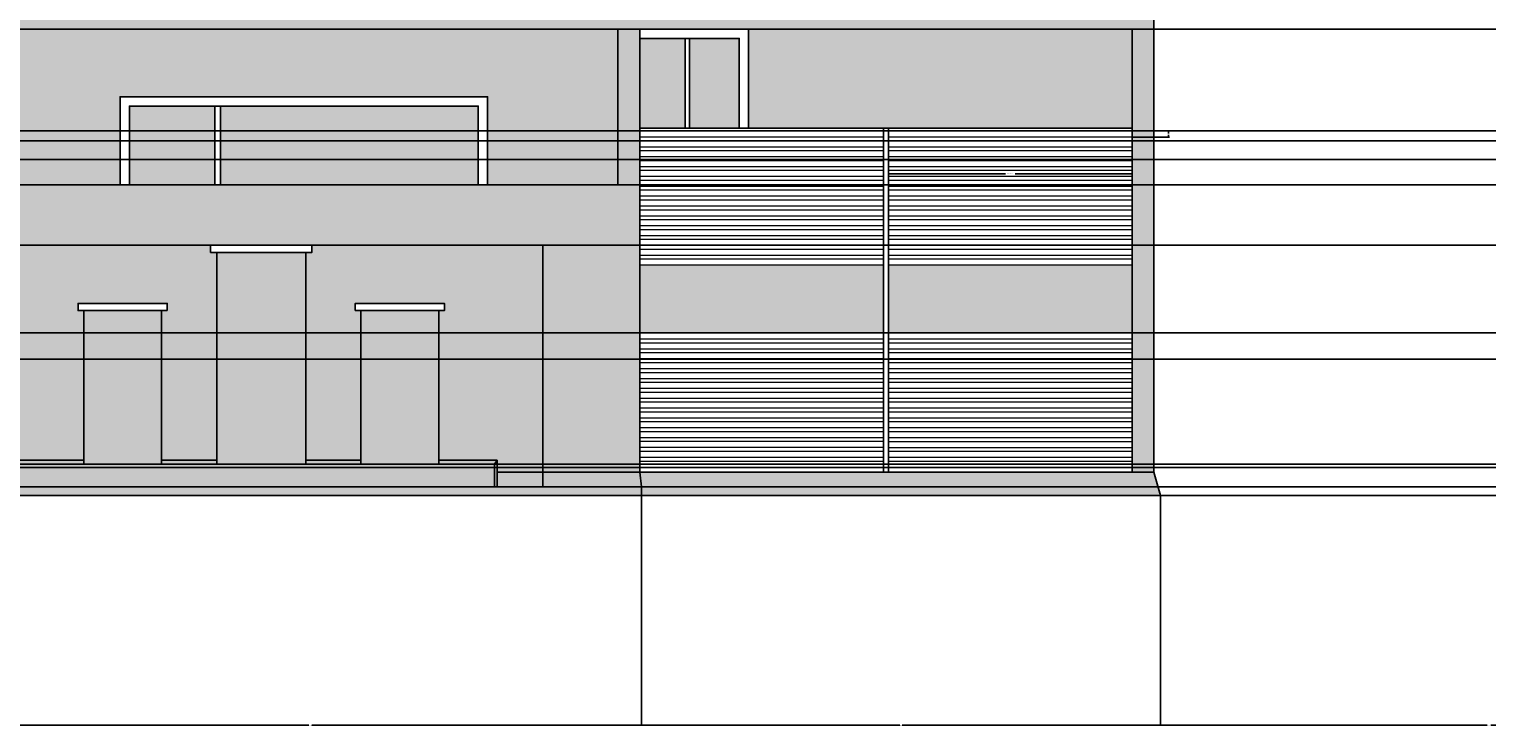
# Model space of a CAD drawing. Units: feet. Extents: x 2193 to 3502, y 890 to 1601.
# Tile 3 of 17: x 2466 to 2848, y 890 to 1073. Entities that reach past the tile are written whole.
import ezdxf

# ---------------------------------------------------------------- set-up
doc = ezdxf.new("R2010")
doc.units = ezdxf.units.FT
for name, color, linetype, lineweight in [('A-ANNO-DIMS', 2, 'Continuous', 18), ('A-ELEV', 7, 'Continuous', 25), ('A-ELEV-GATE', 4, 'Continuous', 18), ('A-ELEV-PATT', 8, 'Continuous', 13)]:
    doc.layers.add(name, color=color, linetype=linetype, lineweight=lineweight)
doc.styles.get("Standard").update_dxf_attribs({"font": 'arial.ttf'})
doc.dimstyles.get("Standard").update_dxf_attribs({"dimtxt": 0.18, "dimasz": 0.18, "dimexe": 0.18, "dimexo": 0.0625, "dimgap": 0.09, "dimtad": 0, "dimtih": 1, "dimtoh": 1, "dimdec": 0, "dimzin": 0, "dimdsep": 46, "dimlunit": 3, "dimtxsty": 'Standard', "dimcen": 0.09, "dimadec": 0, "dimazin": 0, "dimtfac": 1, "dimtdec": 0, "dimtofl": 0, "dimtmove": 0, "dimatfit": 3, "dimfxl": 1, "dimtolj": 1, "dimtzin": 0, "dimarcsym": 0})

# ---------------------------------------------------------------- blocks, each defined once
blk = doc.blocks.new('GATE-SLAT')
blk.add_lwpolyline([(0, 1.66), (63.84, 1.66), (63.84, 0), (0, 0)])
blk.add_lwpolyline([(0, 1.66), (63.84, 1.66), (63.84, 0), (0, 0)])
blk = doc.blocks.new('*D11')
at = {"layer": 'A-ANNO-DIMS', "color": 0, "lineweight": -2, "transparency": 16777216}
for p, q in [((2690.92, 1044.64), (2690.92, 1034.95)), ((2754.77, 1044.64), (2754.77, 1034.95)), ((2691.1, 1035.13), (2721.59, 1035.13)), ((2754.59, 1035.13), (2724.1, 1035.13))]:
    blk.add_line(p, q, dxfattribs=at)
at = {"layer": 'A-ANNO-DIMS', "color": 0, "transparency": 16777216}
for points in [[(2691.1, 1035.16), (2691.1, 1035.1), (2690.92, 1035.13)], [(2754.59, 1035.16), (2754.59, 1035.1), (2754.77, 1035.13)]]:
    blk.add_solid(points, dxfattribs=at)
at = {"layer": 'Defpoints', "color": 0, "transparency": 16777216}
for p in [(2690.92, 1044.7), (2754.77, 1044.7), (2754.77, 1035.13)]:
    blk.add_point(p, dxfattribs=at)
at = {"layer": 'A-ANNO-DIMS', "color": 0, "transparency": 16777216, "insert": (2722.84, 1035.13), "char_height": 0.18, "attachment_point": 5}
blk.add_mtext('\\A1;GATE SLAT 64 TYP.', dxfattribs=at)
blk = doc.blocks.new('*D12')
at = {"layer": 'A-ANNO-DIMS', "color": 0, "lineweight": -2, "transparency": 16777216}
for p, q in [((2754.83, 1046.36), (2764.52, 1046.36)), ((2754.83, 1044.7), (2764.52, 1044.7)), ((2764.34, 1046.18), (2764.34, 1045.71)), ((2764.34, 1044.88), (2764.34, 1045.35))]:
    blk.add_line(p, q, dxfattribs=at)
at = {"layer": 'A-ANNO-DIMS', "color": 0, "transparency": 16777216}
for points in [[(2764.31, 1046.18), (2764.37, 1046.18), (2764.34, 1046.36)], [(2764.31, 1044.88), (2764.37, 1044.88), (2764.34, 1044.7)]]:
    blk.add_solid(points, dxfattribs=at)
at = {"layer": 'Defpoints', "color": 0, "transparency": 16777216}
for p in [(2754.77, 1046.36), (2754.77, 1044.7), (2764.34, 1046.36)]:
    blk.add_point(p, dxfattribs=at)
at = {"layer": 'A-ANNO-DIMS', "color": 0, "transparency": 16777216, "insert": (2764.34, 1045.53), "char_height": 0.18, "attachment_point": 5}
blk.add_mtext('\\A1;2 TYP.', dxfattribs=at)
blk = doc.blocks.new('*D19')
at = {"layer": 'A-ANNO-DIMS', "color": 0, "lineweight": -2, "transparency": 16777216}
for p, q in [((2934.31, 1073.03), (2193.56, 1073.03)), ((2193.74, 1072.85), (2193.74, 1012.11)), ((2193.74, 951), (2193.74, 1011.75)), ((2934.31, 950.82), (2193.56, 950.82))]:
    blk.add_line(p, q, dxfattribs=at)
at = {"layer": 'A-ANNO-DIMS', "color": 0, "transparency": 16777216}
for points in [[(2193.71, 1072.85), (2193.77, 1072.85), (2193.74, 1073.03)], [(2193.71, 951), (2193.77, 951), (2193.74, 950.82)]]:
    blk.add_solid(points, dxfattribs=at)
at = {"layer": 'Defpoints', "color": 0, "transparency": 16777216}
for p in [(2193.74, 1073.03), (2934.37, 1073.03), (2934.37, 950.82)]:
    blk.add_point(p, dxfattribs=at)
at = {"layer": 'A-ANNO-DIMS', "color": 0, "transparency": 16777216, "insert": (2193.74, 1011.93), "char_height": 0.18, "attachment_point": 5}
blk.add_mtext('\\A1;122.2', dxfattribs=at)
blk = doc.blocks.new('*D23')
at = {"layer": 'A-ANNO-DIMS', "color": 0, "lineweight": -2, "transparency": 16777216}
for p, q in [((2988.24, 1038.87), (2193.56, 1038.87)), ((2193.74, 1038.69), (2193.74, 1012.87)), ((2193.74, 986.69), (2193.74, 1012.51)), ((2985.8, 986.51), (2193.56, 986.51))]:
    blk.add_line(p, q, dxfattribs=at)
at = {"layer": 'A-ANNO-DIMS', "color": 0, "transparency": 16777216}
for points in [[(2193.71, 1038.69), (2193.77, 1038.69), (2193.74, 1038.87)], [(2193.71, 986.69), (2193.77, 986.69), (2193.74, 986.51)]]:
    blk.add_solid(points, dxfattribs=at)
at = {"layer": 'Defpoints', "color": 0, "transparency": 16777216}
for p in [(2193.74, 1038.87), (2988.31, 1038.87), (2985.86, 986.51)]:
    blk.add_point(p, dxfattribs=at)
at = {"layer": 'A-ANNO-DIMS', "color": 0, "transparency": 16777216, "insert": (2193.74, 1012.69), "char_height": 0.18, "attachment_point": 5}
blk.add_mtext('\\A1;52.35', dxfattribs=at)
blk = doc.blocks.new('*D26')
at = {"layer": 'A-ANNO-DIMS', "color": 0, "lineweight": -2, "transparency": 16777216}
for p, q in [((2255.16, 950.89), (2255.16, 1601.47)), ((2255.34, 1601.29), (2507.42, 1601.29)), ((2760.29, 1601.29), (2508.21, 1601.29)), ((2760.47, 1541.11), (2760.47, 1601.47))]:
    blk.add_line(p, q, dxfattribs=at)
at = {"layer": 'A-ANNO-DIMS', "color": 0, "transparency": 16777216}
for points in [[(2255.34, 1601.32), (2255.34, 1601.26), (2255.16, 1601.29)], [(2760.29, 1601.32), (2760.29, 1601.26), (2760.47, 1601.29)]]:
    blk.add_solid(points, dxfattribs=at)
at = {"layer": 'Defpoints', "color": 0, "transparency": 16777216}
for p in [(2760.47, 1601.29), (2760.47, 1541.04), (2255.16, 950.82)]:
    blk.add_point(p, dxfattribs=at)
at = {"layer": 'A-ANNO-DIMS', "color": 0, "transparency": 16777216, "insert": (2507.82, 1601.29), "char_height": 0.18, "attachment_point": 5}
blk.add_mtext('\\A1;505.3', dxfattribs=at)
blk = doc.blocks.new('*D29')
at = {"layer": 'A-ANNO-DIMS', "color": 0, "lineweight": -2, "transparency": 16777216}
for p, q in [((2452.78, 956.87), (2452.78, 890.39)), ((2626.2, 950.76), (2626.2, 890.39)), ((2452.96, 890.57), (2539.1, 890.57)), ((2626.02, 890.57), (2539.87, 890.57))]:
    blk.add_line(p, q, dxfattribs=at)
at = {"layer": 'A-ANNO-DIMS', "color": 0, "transparency": 16777216}
for points in [[(2452.96, 890.6), (2452.96, 890.54), (2452.78, 890.57)], [(2626.02, 890.6), (2626.02, 890.54), (2626.2, 890.57)]]:
    blk.add_solid(points, dxfattribs=at)
at = {"layer": 'Defpoints', "color": 0, "transparency": 16777216}
for p in [(2452.78, 956.94), (2626.2, 950.82), (2626.2, 890.57)]:
    blk.add_point(p, dxfattribs=at)
at = {"layer": 'A-ANNO-DIMS', "color": 0, "transparency": 16777216, "insert": (2539.49, 890.57), "char_height": 0.18, "attachment_point": 5}
blk.add_mtext('\\A1;173.4', dxfattribs=at)
blk = doc.blocks.new('*D30')
at = {"layer": 'A-ANNO-DIMS', "color": 0, "lineweight": -2, "transparency": 16777216}
for p, q in [((2626.2, 950.76), (2626.2, 890.39)), ((2762.2, 950.76), (2762.2, 890.39)), ((2626.38, 890.57), (2693.92, 890.57)), ((2762.02, 890.57), (2694.48, 890.57))]:
    blk.add_line(p, q, dxfattribs=at)
at = {"layer": 'A-ANNO-DIMS', "color": 0, "transparency": 16777216}
for points in [[(2626.38, 890.6), (2626.38, 890.54), (2626.2, 890.57)], [(2762.02, 890.6), (2762.02, 890.54), (2762.2, 890.57)]]:
    blk.add_solid(points, dxfattribs=at)
at = {"layer": 'Defpoints', "color": 0, "transparency": 16777216}
for p in [(2626.2, 950.82), (2762.2, 950.82), (2762.2, 890.57)]:
    blk.add_point(p, dxfattribs=at)
at = {"layer": 'A-ANNO-DIMS', "color": 0, "transparency": 16777216, "insert": (2694.2, 890.57), "char_height": 0.18, "attachment_point": 5}
blk.add_mtext('\\A1;136', dxfattribs=at)
blk = doc.blocks.new('*D31')
at = {"layer": 'A-ANNO-DIMS', "color": 0, "lineweight": -2, "transparency": 16777216}
for p, q in [((2760.54, 1541.04), (3501.85, 1541.04)), ((3501.67, 1540.86), (3501.67, 1246.12)), ((3501.67, 951), (3501.67, 1245.75)), ((2762.27, 950.82), (3501.85, 950.82))]:
    blk.add_line(p, q, dxfattribs=at)
at = {"layer": 'A-ANNO-DIMS', "color": 0, "transparency": 16777216}
for points in [[(3501.64, 1540.86), (3501.7, 1540.86), (3501.67, 1541.04)], [(3501.64, 951), (3501.7, 951), (3501.67, 950.82)]]:
    blk.add_solid(points, dxfattribs=at)
at = {"layer": 'Defpoints', "color": 0, "transparency": 16777216}
for p in [(2760.47, 1541.04), (3501.67, 1541.04), (2762.2, 950.82)]:
    blk.add_point(p, dxfattribs=at)
at = {"layer": 'A-ANNO-DIMS', "color": 0, "transparency": 16777216, "insert": (3501.67, 1245.93), "char_height": 0.18, "attachment_point": 5}
blk.add_mtext('\\A1;590.2', dxfattribs=at)
blk = doc.blocks.new('*D98')
at = {"layer": 'A-ANNO-DIMS', "color": 0, "lineweight": -2, "transparency": 16777216}
for p, q in [((3111.07, 1032.19), (2193.56, 1032.19)), ((2193.74, 1032.01), (2193.74, 1024.48)), ((2193.74, 1016.58), (2193.74, 1024.11)), ((3111.07, 1016.4), (2193.56, 1016.4))]:
    blk.add_line(p, q, dxfattribs=at)
at = {"layer": 'A-ANNO-DIMS', "color": 0, "transparency": 16777216}
for points in [[(2193.71, 1032.01), (2193.77, 1032.01), (2193.74, 1032.19)], [(2193.71, 1016.58), (2193.77, 1016.58), (2193.74, 1016.4)]]:
    blk.add_solid(points, dxfattribs=at)
at = {"layer": 'Defpoints', "color": 0, "transparency": 16777216}
for p in [(2193.74, 1032.19), (3111.13, 1032.19), (3111.13, 1016.4)]:
    blk.add_point(p, dxfattribs=at)
at = {"layer": 'A-ANNO-DIMS', "color": 0, "transparency": 16777216, "insert": (2193.74, 1024.3), "char_height": 0.18, "attachment_point": 5}
blk.add_mtext('\\A1;15.793', dxfattribs=at)
blk = doc.blocks.new('*D116')
at = {"layer": 'A-ANNO-DIMS', "color": 0, "lineweight": -2, "transparency": 16777216}
for p, q in [((3140.16, 958.96), (2193.56, 958.96)), ((2193.74, 958.78), (2193.74, 956.18)), ((2193.74, 953.21), (2193.74, 955.81)), ((3140.16, 953.03), (2193.56, 953.03))]:
    blk.add_line(p, q, dxfattribs=at)
at = {"layer": 'A-ANNO-DIMS', "color": 0, "transparency": 16777216}
for points in [[(2193.71, 958.78), (2193.77, 958.78), (2193.74, 958.96)], [(2193.71, 953.21), (2193.77, 953.21), (2193.74, 953.03)]]:
    blk.add_solid(points, dxfattribs=at)
at = {"layer": 'Defpoints', "color": 0, "transparency": 16777216}
for p in [(2193.74, 958.96), (3140.22, 958.96), (3140.22, 953.03)]:
    blk.add_point(p, dxfattribs=at)
at = {"layer": 'A-ANNO-DIMS', "color": 0, "transparency": 16777216, "insert": (2193.74, 955.99), "char_height": 0.18, "attachment_point": 5}
blk.add_mtext('\\A1;5.924', dxfattribs=at)
blk = doc.blocks.new('*D124')
at = {"layer": 'A-ANNO-DIMS', "color": 0, "lineweight": -2, "transparency": 16777216}
for p, q in [((3304.91, 1046.36), (2193.56, 1046.36)), ((3304.91, 1043.78), (2193.56, 1043.78)), ((2193.74, 1046.18), (2193.74, 1045.26)), ((2193.74, 1043.96), (2193.74, 1044.89))]:
    blk.add_line(p, q, dxfattribs=at)
at = {"layer": 'A-ANNO-DIMS', "color": 0, "transparency": 16777216}
for points in [[(2193.71, 1046.18), (2193.77, 1046.18), (2193.74, 1046.36)], [(2193.71, 1043.96), (2193.77, 1043.96), (2193.74, 1043.78)]]:
    blk.add_solid(points, dxfattribs=at)
at = {"layer": 'Defpoints', "color": 0, "transparency": 16777216}
for p in [(2193.74, 1043.78), (3304.97, 1046.36), (3304.97, 1043.78)]:
    blk.add_point(p, dxfattribs=at)
at = {"layer": 'A-ANNO-DIMS', "color": 0, "transparency": 16777216, "insert": (2193.74, 1045.07), "char_height": 0.18, "attachment_point": 5}
blk.add_mtext('\\A1;2.583', dxfattribs=at)
blk = doc.blocks.new('*D126')
at = {"layer": 'A-ANNO-DIMS', "color": 0, "lineweight": -2, "transparency": 16777216}
for p, q in [((2762.2, 950.76), (2762.2, 890.39)), ((2934.37, 950.76), (2934.37, 890.39)), ((2762.38, 890.57), (2847.83, 890.57)), ((2934.19, 890.57), (2848.74, 890.57))]:
    blk.add_line(p, q, dxfattribs=at)
at = {"layer": 'A-ANNO-DIMS', "color": 0, "transparency": 16777216}
for points in [[(2762.38, 890.6), (2762.38, 890.54), (2762.2, 890.57)], [(2934.19, 890.6), (2934.19, 890.54), (2934.37, 890.57)]]:
    blk.add_solid(points, dxfattribs=at)
at = {"layer": 'Defpoints', "color": 0, "transparency": 16777216}
for p in [(2762.2, 950.82), (2934.37, 950.82), (2934.37, 890.57)]:
    blk.add_point(p, dxfattribs=at)
at = {"layer": 'A-ANNO-DIMS', "color": 0, "transparency": 16777216, "insert": (2848.29, 890.57), "char_height": 0.18, "attachment_point": 5}
blk.add_mtext('\\A1;172.17', dxfattribs=at)
blk = doc.blocks.new('*D130')
at = {"layer": 'A-ANNO-DIMS', "color": 0, "lineweight": -2, "transparency": 16777216}
for p, q in [((3304.91, 993.39), (2193.56, 993.39)), ((2193.74, 993.21), (2193.74, 975.95)), ((2193.74, 958.33), (2193.74, 975.59)), ((3304.91, 958.15), (2193.56, 958.15))]:
    blk.add_line(p, q, dxfattribs=at)
at = {"layer": 'A-ANNO-DIMS', "color": 0, "transparency": 16777216}
for points in [[(2193.71, 993.21), (2193.77, 993.21), (2193.74, 993.39)], [(2193.71, 958.33), (2193.77, 958.33), (2193.74, 958.15)]]:
    blk.add_solid(points, dxfattribs=at)
at = {"layer": 'Defpoints', "color": 0, "transparency": 16777216}
for p in [(2193.74, 993.39), (3304.97, 993.39), (3304.97, 958.15)]:
    blk.add_point(p, dxfattribs=at)
at = {"layer": 'A-ANNO-DIMS', "color": 0, "transparency": 16777216, "insert": (2193.74, 975.77), "char_height": 0.18, "attachment_point": 5}
blk.add_mtext('\\A1;35.24', dxfattribs=at)

msp = doc.modelspace()

# ---------------------------------------------------------------- hatches: boundary and pattern name
at = {"layer": 'A-ELEV-PATT'}
h = msp.add_hatch(color=256, dxfattribs=at)
h.dxf.hatch_style = 1
h.paths.add_polyline_path([(2760.4733, 1541.0441), (2699.6322, 1541.0441), (2699.6322, 1512.3957), (2760.4733, 1512.3957)])
h.paths.add_polyline_path([(2760.4733, 1502.0763), (2699.6322, 1502.0763), (2699.6322, 1382.0763), (2760.4733, 1382.0763)])
h.paths.add_polyline_path([(2745.971, 1367.5739), (2699.6322, 1367.5739), (2699.6322, 1089.3627), (2760.4733, 1089.3627), (2760.4733, 1166.2327), (2745.971, 1166.2327)])
h.paths.add_polyline_path([(2754.7661, 1011.1246), (2690.9216, 1011.1246), (2690.9216, 993.3923), (2754.7661, 993.3923)])
h.paths.add_polyline_path([(2689.6008, 1011.1246), (2625.7563, 1011.1246), (2625.7563, 993.3923), (2689.6008, 993.3923)])
h.paths.add_polyline_path([(2599.6883, 1249.8256), (2598.591, 1249.8256), (2598.591, 1233.561), (2599.6883, 1233.561)])
h.paths.add_polyline_path([(2602.5204, 1247.0422), (2601.423, 1247.0422), (2601.423, 1233.561), (2602.5204, 1233.561)])
h.paths.add_polyline_path([(2606.5316, 1250.4403), (2605.4342, 1250.4403), (2605.4342, 1233.561), (2606.5316, 1233.561)])
h.paths.add_polyline_path([(2609.5836, 1248.4363), (2608.4862, 1248.4363), (2608.4862, 1233.561), (2609.5836, 1233.561)])
h.paths.add_polyline_path([(2613.8564, 1243.2956), (2612.759, 1243.2956), (2612.759, 1233.561), (2613.8564, 1233.561)])
h.paths.add_polyline_path([(2616.5596, 1249.6561), (2615.4622, 1249.6561), (2615.4622, 1233.561), (2616.5596, 1233.561)])
h.paths.add_polyline_path([(2599.6883, 1233.561), (2598.591, 1233.561), (2598.591, 1224.865), (2599.6883, 1224.865)])
h.paths.add_polyline_path([(2602.5204, 1233.561), (2601.423, 1233.561), (2601.423, 1224.865), (2602.5204, 1224.865)])
h.paths.add_polyline_path([(2606.5316, 1233.561), (2605.4342, 1233.561), (2605.4342, 1224.865), (2606.5316, 1224.865)])
h.paths.add_polyline_path([(2609.5836, 1233.561), (2608.4862, 1233.561), (2608.4862, 1224.865), (2609.5836, 1224.865)])
h.paths.add_polyline_path([(2613.8564, 1233.561), (2612.759, 1233.561), (2612.759, 1224.865), (2613.8564, 1224.865)])
h.paths.add_polyline_path([(2616.5596, 1233.561), (2615.4622, 1233.561), (2615.4622, 1224.865), (2616.5596, 1224.865)])
h.paths.add_polyline_path([(2599.6883, 1224.865), (2598.591, 1224.865), (2598.591, 1115.2331), (2599.6883, 1115.2331)])
h.paths.add_polyline_path([(2602.5204, 1224.865), (2601.423, 1224.865), (2601.423, 1112.4498), (2602.5204, 1112.4498)])
h.paths.add_polyline_path([(2606.5316, 1224.865), (2605.4342, 1224.865), (2605.4342, 1115.8479), (2606.5316, 1115.8479)])
h.paths.add_polyline_path([(2609.5836, 1224.865), (2608.4862, 1224.865), (2608.4862, 1113.8439), (2609.5836, 1113.8439)])
h.paths.add_polyline_path([(2616.5596, 1224.865), (2615.4622, 1224.865), (2615.4622, 1115.0637), (2616.5596, 1115.0637)])
h.paths.add_polyline_path([(2613.8564, 1224.865), (2612.759, 1224.865), (2612.759, 1108.7032), (2613.8564, 1108.7032)])
h = msp.add_hatch(color=256, dxfattribs=at)
h.dxf.hatch_style = 1
h.paths.add_polyline_path([(2390.8933, 1367.5739), (2294.8992, 1367.5739), (2294.8992, 1329.5765), (2390.8933, 1329.5765)])
h.paths.add_polyline_path([(2489.6169, 1055.3069), (2585.8844, 1055.3069), (2585.8844, 1032.1935), (2620.0491, 1032.1935), (2620.0491, 1073.031), (2452.7821, 1073.031), (2452.7821, 1032.1935), (2489.6169, 1032.1935)])
h.paths.add_polyline_path([(2754.7661, 1073.031), (2654.2841, 1073.031), (2654.2841, 1047.0961), (2754.7661, 1047.0961)])
h.paths.add_polyline_path([(2643.9681, 1484.1152), (2699.5726, 1484.1152), (2699.5726, 1502.0763), (2602.8648, 1502.0763), (2602.8648, 1408.4814), (2643.9681, 1408.4814)])
h.paths.add_polyline_path([(2699.6322, 1367.5739), (2646.2844, 1367.5739), (2646.2844, 1268.6599), (2647.1841, 1268.6599), (2647.1841, 1329.5765), (2699.6322, 1329.5765)])
h.paths.add_polyline_path([(2699.6322, 1224.865), (2616.5596, 1224.865), (2616.5596, 1133.8558), (2647.1841, 1133.8558), (2647.1841, 1194.7724), (2699.6322, 1194.7724)])
h = msp.add_hatch(color=256, dxfattribs=at)
h.dxf.hatch_style = 1
h.paths.add_polyline_path([(2760.4733, 956.8829), (2754.7661, 956.8829), (2625.7563, 956.8829), (2626.1971, 953.031), (2626.1971, 950.8228), (2762.2048, 950.8228)])
h.paths.add_polyline_path([(2587.7084, 958.9555), (2461.0056, 958.9555), (2461.0056, 953.031), (2587.7084, 953.031)])
h.paths.add_polyline_path([(2480.0809, 960.0129), (2463.2716, 960.0129), (2461.0056, 958.9555), (2480.0809, 958.9555)])
h.paths.add_polyline_path([(2514.917, 960.0129), (2500.4779, 960.0129), (2500.4779, 958.9555), (2514.917, 958.9555)])
h.paths.add_polyline_path([(2552.6959, 960.0129), (2538.2568, 960.0129), (2538.2568, 958.9555), (2552.6959, 958.9555)])
h.paths.add_polyline_path([(2588.4279, 960.0129), (2573.0929, 960.0129), (2573.0929, 958.9555), (2587.7084, 958.9555)])
h.paths.add_polyline_path([(2588.4279, 960.0129), (2587.7084, 958.9555), (2587.7084, 953.031), (2588.4279, 953.031)])
h.paths.add_polyline_path([(2461.0056, 956.8829), (2261.443, 956.8829), (2255.1574, 953.031), (2461.0056, 953.031)])
h.paths.add_polyline_path([(2625.7563, 956.8829), (2600.3918, 956.8829), (2600.3918, 953.031), (2626.1971, 953.031)])
h.paths.add_polyline_path([(2600.3918, 956.8829), (2588.4279, 956.8829), (2588.4279, 953.031), (2600.3918, 953.031)])
h.paths.add_polyline_path([(2602.8648, 1494.8043), (2286.5029, 1494.8043), (2286.5029, 1492.5146), (2602.8648, 1492.5146)])
h.paths.add_polyline_path([(2322.8578, 1492.5146), (2319.4392, 1492.5146), (2337.7496, 1475.8561), (2341.1681, 1475.8561)])
h.paths.add_polyline_path([(2341.1681, 1475.8561), (2337.7496, 1475.8561), (2341.051, 1472.8525), (2344.4696, 1472.8525)])
h.paths.add_polyline_path([(2344.4696, 1472.8525), (2341.051, 1472.8525), (2352.3124, 1462.6071), (2355.731, 1462.6071)])
h.paths.add_polyline_path([(2355.731, 1462.6071), (2352.3124, 1462.6071), (2355.6139, 1459.6035), (2359.0325, 1459.6035)])
h.paths.add_polyline_path([(2325.1721, 1459.1592), (2323.1659, 1459.1592), (2323.1659, 1408.4814), (2325.1721, 1408.4814)])
h.paths.add_polyline_path([(2297.6937, 1482.3334), (2295.7368, 1484.1138), (2295.7368, 1408.4814), (2297.6937, 1408.4814)])
h.paths.add_polyline_path([(2300.8766, 1479.4377), (2297.6937, 1482.3334), (2297.6937, 1408.4814), (2300.8766, 1408.4814)])
h.paths.add_polyline_path([(2337.7496, 1475.8561), (2304.8133, 1475.8561), (2308.1148, 1472.8525), (2341.051, 1472.8525)])
h.paths.add_polyline_path([(2352.3124, 1462.6071), (2319.3762, 1462.6071), (2322.6776, 1459.6035), (2355.6139, 1459.6035)])
h.paths.add_polyline_path([(2374.1044, 1475.8561), (2341.1681, 1475.8561), (2344.4696, 1472.8525), (2377.4059, 1472.8525)])
h.paths.add_polyline_path([(2388.6672, 1462.6071), (2355.731, 1462.6071), (2359.0325, 1459.6035), (2391.9687, 1459.6035)])
h.paths.add_polyline_path([(2392.0858, 1462.6071), (2388.6672, 1462.6071), (2391.9687, 1459.6035), (2395.3873, 1459.6035)])
h.paths.add_polyline_path([(2380.8245, 1472.8525), (2377.4059, 1472.8525), (2388.6672, 1462.6071), (2392.0858, 1462.6071)])
h.paths.add_polyline_path([(2377.523, 1475.8561), (2374.1044, 1475.8561), (2377.4059, 1472.8525), (2380.8245, 1472.8525)])
h.paths.add_polyline_path([(2359.2126, 1492.5146), (2355.794, 1492.5146), (2374.1044, 1475.8561), (2377.523, 1475.8561)])
h.paths.add_polyline_path([(2395.5674, 1492.5146), (2392.1488, 1492.5146), (2410.4592, 1475.8561), (2413.8778, 1475.8561)])
h.paths.add_polyline_path([(2410.4592, 1475.8561), (2377.523, 1475.8561), (2380.8245, 1472.8525), (2413.7607, 1472.8525)])
h.paths.add_polyline_path([(2413.8778, 1475.8561), (2410.4592, 1475.8561), (2413.7607, 1472.8525), (2417.1793, 1472.8525)])
h.paths.add_polyline_path([(2417.1793, 1472.8525), (2413.7607, 1472.8525), (2425.022, 1462.6071), (2428.4406, 1462.6071)])
h.paths.add_polyline_path([(2425.022, 1462.6071), (2392.0858, 1462.6071), (2395.3873, 1459.6035), (2428.3235, 1459.6035)])
h.paths.add_polyline_path([(2428.4406, 1462.6071), (2425.022, 1462.6071), (2428.3235, 1459.6035), (2431.7421, 1459.6035)])
h.paths.add_polyline_path([(2461.3769, 1462.6071), (2428.4406, 1462.6071), (2431.7421, 1459.6035), (2464.6784, 1459.6035)])
h.paths.add_polyline_path([(2577.3415, 1492.5146), (2573.9229, 1492.5146), (2591.9256, 1476.1361), (2593.2177, 1478.0707)])
h.paths.add_polyline_path([(2540.9867, 1492.5146), (2537.5681, 1492.5146), (2555.8785, 1475.8561), (2559.2971, 1475.8561)])
h.paths.add_polyline_path([(2591.7386, 1475.8561), (2559.2971, 1475.8561), (2562.5986, 1472.8525), (2589.7325, 1472.8525)])
h.paths.add_polyline_path([(2555.8785, 1475.8561), (2522.9423, 1475.8561), (2526.2437, 1472.8525), (2559.18, 1472.8525)])
h.paths.add_polyline_path([(2559.2971, 1475.8561), (2555.8785, 1475.8561), (2559.18, 1472.8525), (2562.5986, 1472.8525)])
h.paths.add_polyline_path([(2562.5986, 1472.8525), (2559.18, 1472.8525), (2570.4413, 1462.6071), (2573.8599, 1462.6071)])
h.paths.add_polyline_path([(2570.4413, 1462.6071), (2537.5051, 1462.6071), (2540.8066, 1459.6035), (2573.7428, 1459.6035)])
h.paths.add_polyline_path([(2582.8896, 1462.6071), (2573.8599, 1462.6071), (2577.1614, 1459.6035), (2580.8835, 1459.6035)])
h.paths.add_polyline_path([(2573.8599, 1462.6071), (2570.4413, 1462.6071), (2573.7428, 1459.6035), (2577.1614, 1459.6035)])
h.paths.add_polyline_path([(2591.7386, 1475.8561), (2589.7325, 1472.8525), (2589.7325, 1408.4814), (2591.7386, 1408.4814)])
h.paths.add_polyline_path([(2582.8896, 1462.6071), (2580.8835, 1459.6035), (2580.8835, 1408.4814), (2582.8896, 1408.4814)])
h.paths.add_polyline_path([(2504.6319, 1492.5146), (2501.2133, 1492.5146), (2519.5237, 1475.8561), (2522.9423, 1475.8561)])
h.paths.add_polyline_path([(2534.0865, 1462.6071), (2501.1503, 1462.6071), (2504.4518, 1459.6035), (2537.388, 1459.6035)])
h.paths.add_polyline_path([(2537.5051, 1462.6071), (2534.0865, 1462.6071), (2537.388, 1459.6035), (2540.8066, 1459.6035)])
h.paths.add_polyline_path([(2526.2437, 1472.8525), (2522.8252, 1472.8525), (2534.0865, 1462.6071), (2537.5051, 1462.6071)])
h.paths.add_polyline_path([(2522.9423, 1475.8561), (2519.5237, 1475.8561), (2522.8252, 1472.8525), (2526.2437, 1472.8525)])
h.paths.add_polyline_path([(2519.5237, 1475.8561), (2486.5874, 1475.8561), (2489.8889, 1472.8525), (2522.8252, 1472.8525)])
h.paths.add_polyline_path([(2483.1689, 1475.8561), (2450.2326, 1475.8561), (2453.5341, 1472.8525), (2486.4703, 1472.8525)])
h.paths.add_polyline_path([(2486.5874, 1475.8561), (2483.1689, 1475.8561), (2486.4703, 1472.8525), (2489.8889, 1472.8525)])
h.paths.add_polyline_path([(2468.277, 1492.5146), (2464.8585, 1492.5146), (2483.1689, 1475.8561), (2486.5874, 1475.8561)])
h.paths.add_polyline_path([(2489.8889, 1472.8525), (2486.4703, 1472.8525), (2497.7317, 1462.6071), (2501.1503, 1462.6071)])
h.paths.add_polyline_path([(2497.7317, 1462.6071), (2464.7955, 1462.6071), (2468.0969, 1459.6035), (2501.0332, 1459.6035)])
h.paths.add_polyline_path([(2501.1503, 1462.6071), (2497.7317, 1462.6071), (2501.0332, 1459.6035), (2504.4518, 1459.6035)])
h.paths.add_polyline_path([(2464.7955, 1462.6071), (2461.3769, 1462.6071), (2464.6784, 1459.6035), (2468.0969, 1459.6035)])
h.paths.add_polyline_path([(2453.5341, 1472.8525), (2450.1155, 1472.8525), (2461.3769, 1462.6071), (2464.7955, 1462.6071)])
h.paths.add_polyline_path([(2431.9222, 1492.5146), (2428.5036, 1492.5146), (2446.814, 1475.8561), (2450.2326, 1475.8561)])
h.paths.add_polyline_path([(2446.814, 1475.8561), (2413.8778, 1475.8561), (2417.1793, 1472.8525), (2450.1155, 1472.8525)])
h.paths.add_polyline_path([(2450.2326, 1475.8561), (2446.814, 1475.8561), (2450.1155, 1472.8525), (2453.5341, 1472.8525)])
h.paths.add_polyline_path([(2407.5925, 1459.1592), (2405.5863, 1459.1592), (2405.5863, 1408.4814), (2407.5925, 1408.4814)])
h.paths.add_polyline_path([(2499.2252, 1459.1592), (2497.2191, 1459.1592), (2497.2191, 1408.4814), (2499.2252, 1408.4814)])
h = msp.add_hatch(color=256, dxfattribs=at)
h.dxf.hatch_style = 1
h.paths.add_polyline_path([(2294.8992, 1367.5739), (2275.0482, 1367.5739), (2275.0482, 1382.0763), (2536.5416, 1382.0763), (2536.5416, 1406.15), (2256.3232, 1406.15), (2256.3232, 1089.3627), (2255.1574, 1089.3627), (2255.1574, 1073.031), (2294.8992, 1073.031)])
h.paths.add_polyline_path([(2517.7591, 1241.1967), (2468.2854, 1241.1967), (2468.2854, 1224.865), (2598.591, 1224.865), (2598.591, 1233.561), (2517.7591, 1233.561)])
h.paths.add_polyline_path([(2699.6322, 1241.1967), (2636.5184, 1241.1967), (2636.5184, 1233.561), (2616.5596, 1233.561), (2616.5596, 1224.865), (2699.6322, 1224.865)])
h.paths.add_polyline_path([(2615.4622, 1233.561), (2613.8564, 1233.561), (2613.8564, 1224.865), (2615.4622, 1224.865)])
h.paths.add_polyline_path([(2612.759, 1233.561), (2609.5836, 1233.561), (2609.5836, 1224.865), (2612.759, 1224.865)])
h.paths.add_polyline_path([(2608.4862, 1233.561), (2606.5316, 1233.561), (2606.5316, 1224.865), (2608.4862, 1224.865)])
h.paths.add_polyline_path([(2605.4342, 1233.561), (2602.5204, 1233.561), (2602.5204, 1224.865), (2605.4342, 1224.865)])
h.paths.add_polyline_path([(2601.423, 1233.561), (2599.6883, 1233.561), (2599.6883, 1224.865), (2601.423, 1224.865)])
h.paths.add_polyline_path([(2517.7591, 1089.3627), (2468.2854, 1089.3627), (2468.2854, 1079.031), (2294.8992, 1079.031), (2294.8992, 1073.031), (2390.8933, 1073.031), (2452.7821, 1073.031), (2760.4733, 1073.031), (2760.4733, 1089.3627), (2699.6322, 1089.3627), (2636.5184, 1089.3627), (2636.5184, 1081.7269), (2517.7591, 1081.7269)])
h = msp.add_hatch(color=256, dxfattribs=at)
h.dxf.hatch_style = 1
h.paths.add_polyline_path([(2576.3428, 1407.7384), (2536.5416, 1407.7384), (2536.5416, 1406.15), (2536.5416, 1382.0763), (2576.3428, 1382.0763)])
h.paths.add_polyline_path([(2627.3548, 1407.7384), (2576.5924, 1407.7384), (2576.5924, 1382.0763), (2627.3548, 1382.0763)])
h.paths.add_polyline_path([(2667.9236, 1407.7384), (2627.6045, 1407.7384), (2627.6045, 1382.0763), (2667.9236, 1382.0763)])
h.paths.add_polyline_path([(2699.6322, 1407.7384), (2668.1733, 1407.7384), (2668.1733, 1382.0763), (2699.6322, 1382.0763)])
h.paths.add_polyline_path([(2497.5717, 1323.2248), (2470.7305, 1323.2248), (2470.7305, 1271.105), (2497.5717, 1271.105)])
h.paths.add_polyline_path([(2577.3219, 1323.2248), (2500.599, 1323.2248), (2500.599, 1271.105), (2577.3219, 1271.105)])
h.paths.add_polyline_path([(2388.4482, 1327.1314), (2343.4244, 1327.1314), (2343.4244, 1268.6599), (2388.4482, 1268.6599)])
h.paths.add_polyline_path([(2342.3682, 1327.1314), (2297.3443, 1327.1314), (2297.3443, 1268.6599), (2342.3682, 1268.6599)])
h.paths.add_polyline_path([(2335.8632, 1214.8367), (2301.4984, 1214.8367), (2301.4984, 1133.1367), (2335.8632, 1133.1367)])
h.paths.add_polyline_path([(2371.1246, 1214.8367), (2337.2323, 1214.8367), (2337.2323, 1133.1367), (2371.1246, 1133.1367)])
h.paths.add_polyline_path([(2390.8933, 1214.8367), (2372.4936, 1214.8367), (2372.4936, 1133.1367), (2390.8933, 1133.1367)])
h.paths.add_polyline_path([(2577.3219, 1188.4208), (2500.599, 1188.4208), (2500.599, 1136.3009), (2577.3219, 1136.3009)])
h.paths.add_polyline_path([(2497.5717, 1188.4208), (2470.7305, 1188.4208), (2470.7305, 1136.3009), (2497.5717, 1136.3009)])
h.paths.add_polyline_path([(2381.4675, 1132.3937), (2301.4984, 1132.3937), (2301.4984, 1085.6301), (2381.4675, 1085.6301)])
h.paths.add_polyline_path([(2461.6863, 1132.3937), (2381.7172, 1132.3937), (2381.7172, 1085.6301), (2461.6863, 1085.6301)])
h.paths.add_polyline_path([(2494.0463, 1133.1128), (2468.2854, 1133.1128), (2468.2854, 1089.3627), (2494.0463, 1089.3627)])
h.paths.add_polyline_path([(2517.7591, 1133.1128), (2494.296, 1133.1128), (2494.296, 1089.3627), (2517.7591, 1089.3627)])
h.paths.add_polyline_path([(2667.9236, 1133.1128), (2636.5184, 1133.1128), (2636.5184, 1089.3627), (2667.9236, 1089.3627)])
h.paths.add_polyline_path([(2699.6322, 1133.1128), (2668.1733, 1133.1128), (2668.1733, 1089.3627), (2699.6322, 1089.3627)])
h.paths.add_polyline_path([(2651.839, 1070.5859), (2638.7977, 1070.5859), (2638.7977, 1047.0961), (2651.839, 1047.0961)])
h.paths.add_polyline_path([(2637.6317, 1070.5859), (2625.7563, 1070.5859), (2625.7563, 1047.0961), (2637.6317, 1047.0961)])
h.paths.add_polyline_path([(2583.4393, 1052.8618), (2515.9216, 1052.8618), (2515.9216, 1032.1935), (2583.4393, 1032.1935)])
h.paths.add_polyline_path([(2514.4293, 1052.8618), (2492.062, 1052.8618), (2492.062, 1032.1935), (2514.4293, 1032.1935)])
h.paths.add_polyline_path([(2388.4482, 1038.8658), (2348.7682, 1038.8658), (2348.7682, 988.9597), (2388.4482, 988.9597)])
h.paths.add_polyline_path([(2346.3231, 1038.8658), (2309.0883, 1038.8658), (2309.0883, 988.9597), (2346.3231, 988.9597)])
h.paths.add_polyline_path([(2667.9236, 1267.9169), (2636.5184, 1267.9169), (2636.5184, 1241.1967), (2667.9236, 1241.1967)])
h.paths.add_polyline_path([(2699.6322, 1267.9169), (2668.1733, 1267.9169), (2668.1733, 1241.1967), (2699.6322, 1241.1967)])
h.paths.add_polyline_path([(2517.7591, 1267.9169), (2494.296, 1267.9169), (2494.296, 1241.1967), (2517.7591, 1241.1967)])
h.paths.add_polyline_path([(2494.0463, 1267.9169), (2468.2854, 1267.9169), (2468.2854, 1266.7092), (2468.2854, 1241.1967), (2494.0463, 1241.1967)])
h = msp.add_hatch(color=256, dxfattribs=at)
h.dxf.hatch_style = 1
h.paths.add_polyline_path([(2760.4733, 1073.031), (2754.7661, 1073.031), (2754.7661, 956.8829), (2760.4733, 956.8829)])
h.paths.add_polyline_path([(2625.7563, 1073.031), (2620.0491, 1073.031), (2620.0491, 1032.1935), (2625.7563, 1032.1935), (2625.7563, 1047.0961)])
h.paths.add_polyline_path([(2260.8647, 1073.031), (2255.1574, 1073.031), (2255.1574, 953.031), (2260.8647, 956.5285)])
h = msp.add_hatch(color=256, dxfattribs=at)
h.dxf.hatch_style = 1
h.paths.add_polyline_path([(2625.7563, 1032.1935), (2431.9134, 1032.1935), (2431.9134, 1016.4), (2600.3918, 1016.4), (2600.3918, 956.8829), (2625.7563, 956.8829)])
h = msp.add_hatch(color=256, dxfattribs=at)
h.dxf.hatch_style = 1
h.paths.add_polyline_path([(2514.917, 1014.5106), (2513.3297, 1014.5106), (2513.3297, 1016.4), (2452.7821, 1016.4), (2452.7821, 956.8829), (2461.0056, 956.8829), (2461.0056, 958.9555), (2463.2716, 960.0129), (2480.0809, 960.0129), (2480.0809, 999.2439), (2478.6095, 999.2439), (2478.6095, 1001.1334), (2501.9493, 1001.1334), (2501.9493, 999.2439), (2500.4779, 999.2439), (2500.4779, 960.0129), (2514.917, 960.0129)])
h.paths.add_polyline_path([(2552.6959, 999.2439), (2551.2245, 999.2439), (2551.2245, 1001.1334), (2574.5643, 1001.1334), (2574.5643, 999.2439), (2573.0929, 999.2439), (2573.0929, 958.9555), (2587.7084, 958.9555), (2587.7084, 953.031), (2600.3918, 953.031), (2600.3918, 1016.4), (2539.8441, 1016.4), (2539.8441, 1014.5106), (2538.2568, 1014.5106), (2538.2568, 960.0129), (2552.6959, 960.0129)])
h = msp.add_hatch(color=256, dxfattribs=at)
h.dxf.hatch_style = 1
h.paths.add_polyline_path([(2538.2568, 1014.5106), (2514.917, 1014.5106), (2514.917, 958.9555), (2538.2568, 958.9555)])
h.paths.add_polyline_path([(2573.0929, 999.2439), (2552.6959, 999.2439), (2552.6959, 958.9555), (2573.0929, 958.9555)])
h.paths.add_polyline_path([(2500.4779, 999.2439), (2480.0809, 999.2439), (2480.0809, 958.9555), (2500.4779, 958.9555)])
h = msp.add_hatch(color=256, dxfattribs=at)
h.dxf.hatch_style = 1
h.paths.add_polyline_path([(2626.1971, 953.031), (2255.1574, 953.031), (2255.1574, 950.8228), (2626.1971, 950.8228)])

# ---------------------------------------------------------------- linework, layer by layer
at = {"layer": 'A-ELEV'}
for p, q in [((2760.4733, 956.8829), (2760.4733, 1494.0584)), ((2255.1574, 1073.031), (2760.4733, 1073.031)), ((2513.3297, 1016.4), (2513.3297, 1014.5106)), ((2539.8441, 1016.4), (2539.8441, 1014.5106)), ((2463.2716, 960.0129), (2480.0809, 960.0129)), ((2500.4779, 960.0129), (2514.917, 960.0129)), ((2500.4779, 960.0129), (2514.917, 960.0129)), ((2538.2568, 960.0129), (2552.6959, 960.0129)), ((2538.2568, 960.0129), (2552.6959, 960.0129)), ((2573.0929, 960.0129), (2588.4279, 960.0129)), ((2573.0929, 960.0129), (2588.4279, 960.0129)), ((2587.7084, 958.9555), (2588.4279, 960.0129)), ((2588.4279, 960.0129), (2588.4279, 953.031)), ((2588.4279, 956.8829), (2625.7563, 956.8829)), ((2626.1971, 953.031), (2625.7563, 956.8829)), ((2760.4733, 956.8829), (2762.2048, 950.8228)), ((2255.1574, 953.031), (2626.1971, 953.031)), ((2626.1971, 950.8228), (2626.1971, 953.031)), ((2255.1574, 950.8228), (2626.1971, 950.8228)), ((2626.1971, 950.8228), (2762.2048, 950.8228))]:
    msp.add_line(p, q, dxfattribs=at)
for points in [[(2760.4733, 1494.0584), (2760.4733, 956.8829), (2762.2048, 950.8228), (2626.1971, 950.8228), (2255.1574, 950.8228), (2255.1574, 953.031), (2255.1574, 1073.031), (2260.8647, 1073.031), (2260.8647, 956.5285)], [(2255.1574, 1073.031), (2760.4733, 1073.031), (2760.4733, 956.8829), (2754.7661, 956.8829), (2754.7661, 1073.031)], [(2626.1971, 953.031), (2255.1574, 953.031), (2255.1574, 1073.031), (2390.8933, 1073.031), (2390.8933, 956.9371), (2390.8933, 1073.031), (2452.7821, 1073.031), (2452.7821, 1032.1935)], [(2600.3918, 953.031), (2600.3918, 1016.4), (2431.9134, 1016.4), (2431.9134, 1032.1935), (2625.7563, 1032.1935), (2625.7563, 956.8829), (2625.7563, 1073.031), (2620.0491, 1073.031), (2620.0491, 1032.1935)], [(2620.0491, 1032.1935), (2620.0491, 1073.031), (2625.7563, 1073.031), (2625.7563, 956.8829)], [(2625.7563, 1070.5859), (2651.839, 1070.5859), (2651.839, 1047.0961)], [(2625.7563, 1070.5859), (2651.839, 1070.5859), (2651.839, 1047.0961)], [(2760.4733, 1073.031), (2760.4733, 956.8829), (2754.7661, 956.8829), (2754.7661, 1073.031)], [(2492.062, 1032.1935), (2492.062, 1052.8618), (2583.4393, 1052.8618), (2583.4393, 1032.1935)], [(2492.062, 1032.1935), (2492.062, 1052.8618), (2583.4393, 1052.8618), (2583.4393, 1032.1935)], [(2689.6008, 956.8829), (2689.6008, 1047.0961), (2690.9216, 1047.0961), (2690.9216, 956.8829)], [(2689.6008, 956.8829), (2689.6008, 1047.0961), (2690.9216, 1047.0961), (2690.9216, 956.8829)], [(2431.9134, 1016.4), (2431.9134, 1032.1935), (2625.7563, 1032.1935), (2625.7563, 956.8829)], [(2600.3918, 953.031), (2600.3918, 1016.4), (2431.9134, 1016.4)], [(2513.3297, 1016.4), (2539.8441, 1016.4)], [(2539.8441, 1014.5106), (2513.3297, 1014.5106)], [(2514.917, 958.9555), (2514.917, 1014.5106), (2538.2568, 1014.5106), (2538.2568, 958.9555)], [(2514.917, 958.9555), (2514.917, 1014.5106), (2538.2568, 1014.5106), (2538.2568, 958.9555)], [(2480.0809, 958.9555), (2480.0809, 999.2439), (2500.4779, 999.2439), (2500.4779, 958.9555)], [(2480.0809, 958.9555), (2480.0809, 999.2439), (2500.4779, 999.2439), (2500.4779, 958.9555)], [(2573.0929, 958.9555), (2573.0929, 999.2439), (2552.6959, 999.2439), (2552.6959, 958.9555)], [(2573.0929, 958.9555), (2573.0929, 999.2439), (2552.6959, 999.2439), (2552.6959, 958.9555)], [(2461.0056, 958.9555), (2463.2716, 960.0129), (2480.0809, 960.0129)], [(2626.1971, 950.8228), (2626.1971, 953.031), (2625.7563, 956.8829), (2588.4279, 956.8829)]]:
    msp.add_lwpolyline(points, dxfattribs=at)
for points in [[(2625.7563, 1073.031), (2654.2841, 1073.031), (2654.2841, 1047.0961), (2625.7563, 1047.0961)], [(2625.7563, 1073.031), (2654.2841, 1073.031), (2654.2841, 1047.0961), (2625.7563, 1047.0961)], [(2638.7977, 1070.5859), (2637.6317, 1070.5859), (2637.6317, 1047.0961), (2638.7977, 1047.0961)], [(2638.7977, 1070.5859), (2637.6317, 1070.5859), (2637.6317, 1047.0961), (2638.7977, 1047.0961)], [(2585.8844, 1032.1935), (2489.6169, 1032.1935), (2489.6169, 1055.3069), (2585.8844, 1055.3069)], [(2585.8844, 1032.1935), (2489.6169, 1032.1935), (2489.6169, 1055.3069), (2585.8844, 1055.3069)], [(2514.4293, 1052.8618), (2515.9216, 1052.8618), (2515.9216, 1032.1935), (2514.4293, 1032.1935)], [(2514.4293, 1052.8618), (2515.9216, 1052.8618), (2515.9216, 1032.1935), (2514.4293, 1032.1935)], [(2754.7661, 956.8829), (2625.7563, 956.8829), (2625.7563, 1047.0961), (2754.7661, 1047.0961)], [(2754.7661, 956.8829), (2625.7563, 956.8829), (2625.7563, 1047.0961), (2754.7661, 1047.0961)], [(2513.3297, 1014.5106), (2513.3297, 1016.4), (2539.8441, 1016.4), (2539.8441, 1014.5106)], [(2501.9493, 999.2439), (2478.6095, 999.2439), (2478.6095, 1001.1334), (2501.9493, 1001.1334)], [(2501.9493, 999.2439), (2478.6095, 999.2439), (2478.6095, 1001.1334), (2501.9493, 1001.1334)], [(2551.2245, 999.2439), (2574.5643, 999.2439), (2574.5643, 1001.1334), (2551.2245, 1001.1334)], [(2551.2245, 999.2439), (2574.5643, 999.2439), (2574.5643, 1001.1334), (2551.2245, 1001.1334)], [(2461.0056, 953.031), (2587.7084, 953.031), (2587.7084, 958.9555), (2461.0056, 958.9555)], [(2461.0056, 953.031), (2587.7084, 953.031), (2587.7084, 958.9555), (2461.0056, 958.9555)]]:
    msp.add_lwpolyline(points, close=True, dxfattribs=at)

# ---------------------------------------------------------------- block references
at = {"layer": 'A-ELEV-GATE', "rotation": 180}
for p in [(2689.6004, 1046.3647), (2689.6004, 1043.7818), (2689.6004, 1041.1988), (2689.6004, 1038.6159), (2689.6004, 1036.033), (2689.6004, 1033.45), (2689.6004, 1030.8671), (2689.6004, 1028.2842), (2689.6004, 1025.7012), (2689.6004, 1023.1183), (2689.6004, 1020.5354), (2689.6004, 1017.9524), (2689.6004, 1015.3695), (2689.6004, 1012.7866), (2689.6004, 993.3921), (2689.6004, 990.8091), (2689.6004, 988.2262), (2689.6004, 985.6433), (2689.6004, 983.0603), (2689.6004, 980.4774), (2689.6004, 977.8944), (2689.6004, 975.3115), (2689.6004, 972.7286), (2689.6004, 970.1456), (2689.6004, 967.5627), (2689.6004, 964.9798), (2689.6004, 962.3968), (2689.6004, 959.8139)]:
    msp.add_blockref('GATE-SLAT', p, dxfattribs=at)
at = {"layer": 'A-ELEV-GATE'}
for p in [(2690.922, 1044.703), (2690.922, 1042.1201), (2690.922, 1039.5371), (2690.922, 1036.9542), (2690.922, 1034.3713), (2690.922, 1031.7883), (2690.922, 1029.2054), (2690.922, 1026.6225), (2690.922, 1024.0395), (2690.922, 1021.4566), (2690.922, 1018.8736), (2690.922, 1016.2907), (2690.922, 1013.7078), (2690.922, 1011.1248), (2690.922, 991.7303), (2690.922, 989.1474), (2690.922, 986.5645), (2690.922, 983.9815), (2690.922, 981.3986), (2690.922, 978.8157), (2690.922, 976.2327), (2690.922, 973.6498), (2690.922, 971.0669), (2690.922, 968.4839), (2690.922, 965.901), (2690.922, 963.3181), (2690.922, 960.7351), (2690.922, 958.1522)]:
    msp.add_blockref('GATE-SLAT', p, dxfattribs=at)

# ---------------------------------------------------------------- dimensions: what is measured, and where the dimension line sits
at = {"layer": 'A-ANNO-DIMS'}
for base, p1, p2, override, picture, middle in [((2760.4733, 1601.2941), (2255.1574, 950.8228), (2760.4733, 1541.0441), {"dimdec": 1, "dimlfac": 1, "dimrnd": 0, "dimzin": 0, "dimdsep": 46, "dimlunit": 2}, '*D26', (2507.8154, 1601.2941)), ((2626.1971, 890.5728), (2452.7821, 956.9371), (2626.1971, 950.8228), {"dimdec": 1, "dimlfac": 1, "dimrnd": 0, "dimzin": 0, "dimdsep": 46, "dimlunit": 2}, '*D29', (2539.4896, 890.5728)), ((2762.2048, 890.5728), (2626.1971, 950.8228), (2762.2048, 950.8228), {"dimdec": 0, "dimlfac": 1, "dimrnd": 0, "dimzin": 0, "dimdsep": 46, "dimlunit": 2}, '*D30', (2694.201, 890.5728)), ((2934.3742, 890.5728), (2762.2048, 950.8228), (2934.3742, 950.8228), {"dimdec": 2, "dimlfac": 1, "dimrnd": 0, "dimzin": 0, "dimdsep": 46, "dimlunit": 2}, '*D126', (2848.2895, 890.5728))]:
    dim = msp.add_linear_dim(base=base, p1=p1, p2=p2, dimstyle='Standard', override=override, dxfattribs=at)
    dim.commit()
    dim.dimension.update_dxf_attribs({"geometry": picture, "text_midpoint": middle})
for base, p1, p2, override, picture, middle in [((3501.6716, 1541.0441), (2762.2048, 950.8228), (2760.4733, 1541.0441), {"dimdec": 1, "dimlfac": 1, "dimrnd": 0, "dimzin": 0, "dimdsep": 46, "dimlunit": 2}, '*D31', (3501.6716, 1245.9334)), ((2193.7417, 1073.031), (2934.3742, 950.8228), (2934.3742, 1073.031), {"dimdec": 1, "dimlfac": 1, "dimrnd": 0, "dimzin": 0, "dimdsep": 46, "dimlunit": 2}, '*D19', (2193.7417, 1011.9269)), ((2193.7417, 1043.7821), (3304.9731, 1046.365), (3304.9731, 1043.7821), {"dimdec": 3, "dimlfac": 1, "dimrnd": 0, "dimzin": 0, "dimdsep": 46, "dimlunit": 2}, '*D124', (2193.7417, 1045.0735)), ((2193.7417, 1038.8658), (2985.8599, 986.5146), (2988.305, 1038.8658), {"dimdec": 2, "dimlfac": 1, "dimrnd": 0, "dimzin": 0, "dimdsep": 46, "dimlunit": 2}, '*D23', (2193.7417, 1012.6902)), ((2193.7417, 1032.19351), (3111.13015, 1016.40002), (3111.13015, 1032.19351), {"dimdec": 3, "dimlfac": 1, "dimrnd": 0, "dimzin": 0, "dimdsep": 46, "dimlunit": 2}, '*D98', (2193.7417, 1024.29676)), ((2193.7417, 993.3923), (3304.9731, 958.1519), (3304.9731, 993.3923), {"dimdec": 2, "dimlfac": 1, "dimrnd": 0, "dimzin": 0, "dimdsep": 46, "dimlunit": 2}, '*D130', (2193.7417, 975.7721)), ((2193.7417, 958.95546), (3140.22232, 953.03099), (3140.22232, 958.95546), {"dimdec": 3, "dimlfac": 1, "dimrnd": 0, "dimzin": 0, "dimdsep": 46, "dimlunit": 2}, '*D116', (2193.7417, 955.99323))]:
    dim = msp.add_linear_dim(base=base, p1=p1, p2=p2, angle=90, dimstyle='Standard', override=override, dxfattribs=at)
    dim.commit()
    dim.dimension.update_dxf_attribs({"geometry": picture, "text_midpoint": middle})
dim = msp.add_linear_dim(base=(2754.7661, 1035.126), p1=(2690.9216, 1044.7027), p2=(2754.7661, 1044.7027), text='GATE SLAT <> TYP.', dimstyle='Standard', override={"dimdec": 0, "dimlfac": 1, "dimrnd": 0, "dimzin": 0, "dimdsep": 46, "dimlunit": 2}, dxfattribs=at)
dim.commit()
dim.dimension.update_dxf_attribs({"geometry": '*D11', "text_midpoint": (2722.8439, 1035.126)})
dim = msp.add_linear_dim(base=(2764.3428, 1046.365), p1=(2754.7661, 1044.7027), p2=(2754.7661, 1046.365), angle=90, text='<> TYP.', dimstyle='Standard', override={"dimdec": 0, "dimlfac": 1, "dimrnd": 0, "dimzin": 0, "dimdsep": 46, "dimlunit": 2}, dxfattribs=at)
dim.commit()
dim.dimension.update_dxf_attribs({"geometry": '*D12', "text_midpoint": (2764.3428, 1045.5339)})

doc.saveas('drawing.dxf')
